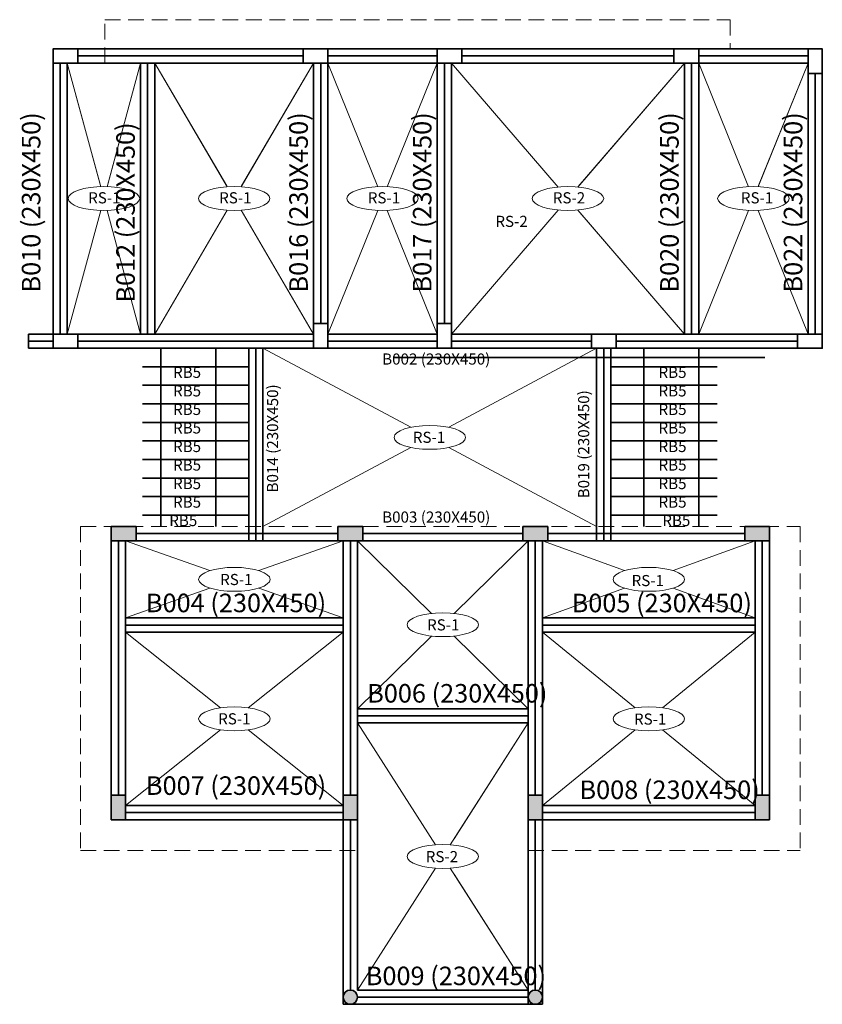
# Model space of a CAD drawing. Units: millimetres. Extents: x 15 to 330868, y -4710 to 1734924.
# Tile 1 of 3: x 280070 to 293056, y 850107 to 866041. Entities that reach past the tile are written whole.
import ezdxf

# ---------------------------------------------------------------- set-up
doc = ezdxf.new("R2010")
doc.units = ezdxf.units.MM
doc.header["$MEASUREMENT"] = 0
doc.linetypes.add('DASHED', pattern=[19.05, 12.7, -6.35])
for name, color, linetype, lineweight in [('S-ANNO-SYMB', 2, 'Continuous', 18), ('S-ANNO-TEXT', 7, 'Continuous', 18), ('S-BEAM', 7, 'Continuous', 35), ('S-COLS', 8, 'Continuous', 35), ('S-SLAB', 8, 'Continuous', 13), ('S-SLAB-OVHD', 6, 'DASHED', 18)]:
    doc.layers.add(name, color=color, linetype=linetype, lineweight=lineweight)
doc.styles.get("Standard").update_dxf_attribs({"font": 'arial.ttf'})

msp = doc.modelspace()

# ---------------------------------------------------------------- hatches: boundary and pattern name
at = {"layer": 'S-COLS'}
h = msp.add_hatch(color=256, dxfattribs=at)
h.dxf.hatch_style = 1
h.paths.add_polyline_path([(288527.5, 853493.6), (288297.5, 853493.6), (288297.5, 853093.6), (288527.5, 853093.6)])
h.paths.add_polyline_path([(285535, 853493.6), (285305, 853493.6), (285305, 853093.6), (285535, 853093.6)])
h.paths.add_polyline_path([(292200.2, 853493.6), (291970.2, 853493.6), (291970.2, 853093.6), (292200.2, 853093.6)])
h.paths.add_polyline_path([(288612.5, 857838.6), (288212.5, 857838.6), (288212.5, 857608.6), (288612.5, 857608.6)])
h.paths.add_polyline_path([(285620, 857838.6), (285220, 857838.6), (285220, 857608.6), (285620, 857608.6)])
h.paths.add_polyline_path([(281952, 857838.6), (281552, 857838.6), (281552, 857608.6), (281952, 857608.6)])
h.paths.add_polyline_path([(281782, 853493.6), (281552, 853493.6), (281552, 853093.6), (281782, 853093.6)])
h = msp.add_hatch(color=256, dxfattribs=at)
h.dxf.hatch_style = 1
h.paths.add_polyline_path([(292200.2, 857838.6), (291800.2, 857838.6), (291800.2, 857608.6), (292200.2, 857608.6)])
h = msp.add_hatch(color=256, dxfattribs=at)
h.dxf.hatch_style = 1
h.paths.add_polyline_path([(288527.5, 850221.5, 1), (288297.5, 850221.5, 1)])
h.paths.add_polyline_path([(285305, 850221.5, 1), (285535, 850221.5, 1)])

# ---------------------------------------------------------------- linework, layer by layer
at = {"layer": 'S-ANNO-SYMB'}
for centre in [(281433.2, 863146.1), (283540.7, 863146.1), (285940.7, 863146.1), (288940.7, 863146.1), (291940.7, 863146.1), (286705.4, 859281.1), (283543.5, 856983.7), (290248.8, 856983.7), (286916.3, 856249.6), (283543.5, 854726.2), (290248.8, 854726.2), (286916.3, 852498.6)]:
    msp.add_ellipse(centre, major_axis=(578.3, 0), ratio=0.3340635, dxfattribs=at)
at = {"layer": 'S-BEAM'}
for p, q in [((280610.7, 865568.6), (280610.7, 860723.6)), ((280610.7, 865568.6), (293055.7, 865568.6)), ((285055.7, 865568.6), (285055.7, 860723.6)), ((286825.7, 865568.6), (286825.7, 860723.6)), ((291055.7, 865568.6), (291055.7, 860953.6)), ((292825.7, 865568.6), (292825.7, 860953.6)), ((293055.7, 865568.6), (293055.7, 860723.6)), ((281010.7, 865453.6), (284655.7, 865453.6)), ((285055.7, 865453.6), (286825.7, 865453.6)), ((287225.7, 865453.6), (290655.7, 865453.6)), ((291055.7, 865453.6), (292825.7, 865453.6)), ((280610.7, 865338.6), (292825.7, 865338.6)), ((280725.7, 860953.6), (280725.7, 865338.6)), ((280840.7, 865338.6), (280840.7, 860953.6)), ((282025.7, 865338.6), (282025.7, 860953.6)), ((282140.7, 865338.6), (282140.7, 860953.6)), ((282255.7, 865338.6), (282255.7, 860953.6)), ((284825.7, 865338.6), (284825.7, 860723.6)), ((284940.7, 865338.6), (284940.7, 861123.6)), ((286940.7, 865338.6), (286940.7, 861123.6)), ((287055.7, 865338.6), (287055.7, 860723.6)), ((290825.7, 865338.6), (290825.7, 860953.6)), ((290940.7, 865338.6), (290940.7, 860953.6)), ((292940.7, 865168.6), (292940.7, 860953.6)), ((280210.7, 860953.6), (284825.7, 860953.6)), ((280210.7, 860953.6), (280210.7, 860723.6)), ((285055.7, 860953.6), (286825.7, 860953.6)), ((287055.7, 860953.6), (293055.7, 860953.6)), ((280610.7, 860838.6), (280210.7, 860838.6)), ((281010.7, 860838.6), (284825.7, 860838.6)), ((285055.7, 860838.6), (286825.7, 860838.6)), ((287055.7, 860838.6), (289319.1, 860838.6)), ((289719.1, 860838.6), (292655.7, 860838.6)), ((280210.7, 860723.6), (293055.7, 860723.6)), ((282354.7, 860723.6), (282354.7, 857838.6)), ((283241.3, 860723.6), (283241.3, 857838.6)), ((283776.6, 860723.6), (283776.6, 857608.6)), ((283891.6, 860723.6), (283891.6, 857608.6)), ((284006.6, 860723.6), (284006.6, 857608.6)), ((289404.1, 860723.6), (289404.1, 857608.6)), ((289519.1, 860723.6), (289519.1, 857608.6)), ((289634.1, 860723.6), (289634.1, 857608.6)), ((290169.2, 860723.6), (290169.2, 857838.6)), ((291055.7, 860723.6), (291055.7, 857838.6)), ((286126.6, 860572.5), (292126.6, 860572.5)), ((283776.4, 860423.6), (282054.7, 860423.6)), ((289634.1, 860423.6), (291355.7, 860423.6)), ((283776.4, 860123.6), (282054.7, 860123.6)), ((289634.1, 860123.6), (291355.7, 860123.6)), ((283776.4, 859823.6), (282054.7, 859823.6)), ((289634.1, 859823.6), (291355.7, 859823.6)), ((283776.4, 859523.6), (282054.7, 859523.6)), ((289634.1, 859523.6), (291355.7, 859523.6)), ((283776.4, 859223.6), (282054.7, 859223.6)), ((289634.1, 859223.6), (291355.7, 859223.6)), ((283776.4, 858923.6), (282054.7, 858923.6)), ((289634.1, 858923.6), (291355.7, 858923.6)), ((283776.4, 858623.6), (282054.7, 858623.6)), ((289634.1, 858623.6), (291355.7, 858623.6)), ((283776.4, 858323.6), (282054.7, 858323.6)), ((289634.1, 858323.6), (291355.7, 858323.6)), ((283776.4, 858023.6), (282054.7, 858023.6)), ((289634.1, 858023.6), (291355.7, 858023.6)), ((281552, 857838.6), (281552, 853093.6)), ((292200.2, 857838.6), (292200.2, 853093.6)), ((281552, 857608.6), (292200.2, 857608.6)), ((281667, 857608.6), (281667, 853493.6)), ((281782, 857608.6), (281782, 853093.6)), ((281952, 857723.6), (285220, 857723.6)), ((285305, 857608.6), (285305, 850106.5)), ((285420, 857608.6), (285420, 853493.6)), ((285535, 857608.6), (285535, 850336.5)), ((285620, 857723.6), (288212.5, 857723.6)), ((288297.5, 857608.6), (288297.5, 850106.5)), ((288412.5, 857608.6), (288412.5, 853493.6)), ((288527.5, 857608.6), (288527.5, 850106.5)), ((288612.5, 857723.6), (291800.2, 857723.6)), ((291970.2, 857608.6), (291970.2, 853093.6)), ((292085.2, 857608.6), (292085.2, 853493.6)), ((281782, 856358.9), (285305, 856358.9)), ((288527.5, 856358.9), (291970.2, 856358.9)), ((281782, 856243.9), (285305, 856243.9)), ((288527.5, 856243.9), (291970.2, 856243.9)), ((281782, 856128.9), (285305, 856128.9)), ((288527.5, 856128.9), (291970.2, 856128.9)), ((285535, 854890.7), (288297.5, 854890.7)), ((285535, 854775.7), (288297.5, 854775.7)), ((285535, 854660.7), (288297.5, 854660.7)), ((281782, 853323.6), (285305, 853323.6)), ((288527.5, 853323.6), (291970.2, 853323.6)), ((281782, 853208.6), (285305, 853208.6)), ((288527.5, 853208.6), (291970.2, 853208.6)), ((281552, 853093.6), (285535, 853093.6)), ((285420, 853093.6), (285420, 850336.5)), ((288297.5, 853093.6), (292200.2, 853093.6)), ((288412.5, 853093.6), (288412.5, 850336.5)), ((285535, 850336.5), (288297.5, 850336.5)), ((285305, 850106.5), (288527.5, 850106.5)), ((285535, 850221.5), (288297.5, 850221.5))]:
    msp.add_line(p, q, dxfattribs=at)
for points in [[(281010.7, 865568.6), (281010.7, 865338.6), (280610.7, 865338.6), (280610.7, 865568.6)], [(285055.7, 865568.6), (285055.7, 865338.6), (284655.7, 865338.6), (284655.7, 865568.6)], [(287225.7, 865568.6), (287225.7, 865338.6), (286825.7, 865338.6), (286825.7, 865568.6)], [(291055.7, 865568.6), (291055.7, 865338.6), (290655.7, 865338.6), (290655.7, 865568.6)], [(292825.7, 865568.6), (293055.7, 865568.6), (293055.7, 865168.6), (292825.7, 865168.6)], [(284825.7, 861123.6), (285055.7, 861123.6), (285055.7, 860723.6), (284825.7, 860723.6)], [(286825.7, 861123.6), (287055.7, 861123.6), (287055.7, 860723.6), (286825.7, 860723.6)], [(281010.7, 860953.6), (281010.7, 860723.6), (280610.7, 860723.6), (280610.7, 860953.6)], [(289719.1, 860953.6), (289719.1, 860723.6), (289319.1, 860723.6), (289319.1, 860953.6)], [(293055.7, 860953.6), (293055.7, 860723.6), (292655.7, 860723.6), (292655.7, 860953.6)], [(281952, 857838.6), (281952, 857608.6), (281552, 857608.6), (281552, 857838.6)], [(285620, 857838.6), (285620, 857608.6), (285220, 857608.6), (285220, 857838.6)], [(288612.5, 857838.6), (288612.5, 857608.6), (288212.5, 857608.6), (288212.5, 857838.6)], [(292200.2, 857838.6), (292200.2, 857608.6), (291800.2, 857608.6), (291800.2, 857838.6)], [(281552, 853493.6), (281782, 853493.6), (281782, 853093.6), (281552, 853093.6)], [(285305, 853493.6), (285535, 853493.6), (285535, 853093.6), (285305, 853093.6)], [(288297.5, 853493.6), (288527.5, 853493.6), (288527.5, 853093.6), (288297.5, 853093.6)], [(291970.2, 853493.6), (292200.2, 853493.6), (292200.2, 853093.6), (291970.2, 853093.6)]]:
    msp.add_lwpolyline(points, close=True, dxfattribs=at)
at = {"layer": 'S-COLS'}
for centre in [(285420, 850221.5), (288412.5, 850221.5)]:
    msp.add_circle(centre, 115, dxfattribs=at)
at = {"layer": 'S-SLAB'}
for p, q in [((281375.7, 863358.9), (280840.7, 865338.6)), ((281381.2, 863338.5), (280840.7, 865338.6)), ((282025.7, 865338.6), (281485.2, 863338.5)), ((282025.7, 865338.6), (281490.8, 863358.9)), ((282255.7, 865338.6), (283421.2, 863350.1)), ((282255.7, 865338.6), (283429.6, 863335.7)), ((283651.9, 863335.7), (284825.7, 865338.6)), ((283660.3, 863350.1), (284825.7, 865338.6)), ((285055.7, 865338.6), (285864.4, 863335.1)), ((286016.3, 863333.3), (286825.7, 865338.6)), ((287055.7, 865338.6), (288781.1, 863331.8)), ((289100.4, 863331.8), (290825.7, 865338.6)), ((289106.4, 863338.8), (290825.7, 865338.6)), ((291055.7, 865338.6), (291863.5, 863337.6)), ((292018, 863337.6), (292825.7, 865338.6)), ((292025.4, 863355.9), (292825.7, 865338.6)), ((281381.2, 862953.7), (280840.7, 860953.6)), ((282025.7, 860953.6), (281485.2, 862953.7)), ((282255.7, 860953.6), (283429.6, 862956.5)), ((283651.9, 862956.5), (284825.7, 860953.6)), ((285055.7, 860953.6), (285863.5, 862954.7)), ((286018, 862954.7), (286825.7, 860953.6)), ((287055.7, 860953.6), (288781.1, 862960.4)), ((289100.4, 862960.4), (290825.7, 860953.6)), ((289106.4, 862953.4), (290825.7, 860953.6)), ((291055.7, 860953.6), (291863.5, 862954.7)), ((292018, 862954.7), (292825.7, 860953.6)), ((284006.6, 860723.6), (286398.9, 859444.9)), ((289404.1, 860723.6), (287011.9, 859444.9)), ((286398.9, 859117.3), (284006.6, 857838.6)), ((287011.9, 859117.3), (289404.1, 857838.6)), ((281782, 857608.6), (283147, 857124.4)), ((283940, 857124.4), (285305, 857608.6)), ((285535, 857608.6), (286730.3, 856432.6)), ((287102.2, 856432.6), (288297.5, 857608.6)), ((289857.3, 857125.9), (288527.5, 857608.6)), ((290640.4, 857125.9), (291970.2, 857608.6)), ((281782, 856358.9), (283147, 856843.1)), ((283940, 856843.1), (285305, 856358.9)), ((288527.5, 856358.9), (289857.3, 856841.6)), ((291970.2, 856358.9), (290640.4, 856841.6)), ((283319.8, 854904.4), (281782, 856128.9)), ((283767.2, 854904.4), (285305, 856128.9)), ((285535, 854890.7), (286730.3, 856066.7)), ((287102.2, 856066.7), (288297.5, 854890.7)), ((288527.5, 856128.9), (290029.5, 854905)), ((291970.2, 856128.9), (290468.2, 854905)), ((285535, 854660.7), (286795.5, 852687.5)), ((287037, 852687.5), (288297.5, 854660.7)), ((287097.5, 852782.4), (288297.5, 854660.7)), ((281782, 853323.6), (283319.8, 854548.1)), ((285305, 853323.6), (283767.2, 854548.1)), ((290029.5, 854547.5), (288527.5, 853323.6)), ((290468.2, 854547.5), (291970.2, 853323.6)), ((285535, 850336.5), (286795.5, 852309.7)), ((287037, 852309.7), (288297.5, 850336.5)), ((287099.9, 852211.2), (288297.5, 850336.5))]:
    msp.add_line(p, q, dxfattribs=at)
at = {"layer": 'S-SLAB-OVHD', "ltscale": 20}
for p, q in [((281445.5, 865338.6), (281445.5, 866040.7)), ((281445.5, 866040.7), (291564.7, 866040.7)), ((291564.7, 866040.7), (291564.7, 865568.6)), ((281052, 857838.6), (292700.2, 857838.6)), ((281052, 857838.6), (281052, 852593.6)), ((292700.2, 857838.6), (292700.2, 852593.6)), ((281052, 852593.6), (285535, 852593.6)), ((288297.5, 852593.6), (292700.2, 852593.6))]:
    msp.add_line(p, q, dxfattribs=at)

# ---------------------------------------------------------------- texts
at = {"layer": 'S-ANNO-TEXT', "attachment_point": 1, "rotation": 90}
for s, width, insert, char_height in [('\\pxt0,1;B010 (230X450)', 4992.481, (280105.1, 861625.9), 300), ('\\pxt0,1;B016 (230X450)', 4992.481, (284432.4, 861625.9), 300), ('\\pxt0,1;B017 (230X450)', 4992.481, (286432.4, 861625.9), 300), ('\\pxt0,1;B020 (230X450)', 4992.481, (290432.4, 861625.9), 300), ('\\pxt0,1;B022 (230X450)', 4992.481, (292432.4, 861625.9), 300), ('\\pxt0,1;B012 (230X450)', 4992.481, (281632.4, 861462.5), 300), ('\\pxt0;B014 (230X450)', 2161.345, (284071.4, 858390.2), 180), ('B019 (230X450)', 2161.345, (289104.9, 858294.7), 180)]:
    msp.add_mtext_dynamic_manual_height_columns(s, width=width, gutter_width=1, heights=[0], dxfattribs=dict(at, insert=insert, char_height=char_height))
at = {"layer": 'S-ANNO-TEXT'}
for s, width, insert, char_height, attachment_point in [('RS-1', 774.454, (281178.2, 863248.3), 180, 1), ('RS-1', 774.454, (283297.3, 863248.3), 180, 1), ('RS-1', 774.454, (285702, 863248.3), 180, 1), ('RS-2', 774.454, (288695.6, 863248.3), 180, 1), ('RS-1', 774.454, (291738, 863248.3), 180, 1), ('RS-2', 774.454, (287766.4, 862867.2), 180, 1), ('B002 (230X450)', 2161.345, (285934.7, 860639.2), 180, 1), ('RB5 ', 774.454, (283005, 860423.6), 180, 3), ('RB5 ', 774.454, (290405.5, 860423.6), 180, 1), ('RB5 ', 774.454, (283005, 860123.6), 180, 3), ('RB5 ', 774.454, (290405.5, 860123.6), 180, 1), ('RB5 ', 774.454, (283005, 859823.6), 180, 3), ('RB5 ', 774.454, (290405.5, 859823.6), 180, 1), ('RB5 ', 774.454, (283005, 859523.6), 180, 3), ('RB5 ', 774.454, (290405.5, 859523.6), 180, 1), ('RS-1', 774.454, (286430.7, 859372.5), 180, 1), ('RB5 ', 774.454, (283005, 859223.6), 180, 3), ('RB5 ', 774.454, (290405.5, 859223.6), 180, 1), ('RB5 ', 774.454, (283005, 858923.6), 180, 3), ('RB5 ', 774.454, (290405.5, 858923.6), 180, 1), ('RB5 ', 774.454, (283005, 858623.6), 180, 3), ('RB5 ', 774.454, (290405.5, 858623.6), 180, 1), ('RB5 ', 774.454, (283005, 858323.6), 180, 3), ('RB5 ', 774.454, (290405.5, 858323.6), 180, 1), ('B003 (230X450)', 2161.345, (285934.7, 858081.8), 180, 1), ('RB5 ', 774.454, (282943.4, 858025.1), 180, 3), ('RB5 ', 774.454, (290467.1, 858025.1), 180, 1), ('RS-1', 774.454, (283313.4, 857071), 180, 1), ('RS-1', 774.454, (289970.6, 857054), 180, 1), ('\\pxt0,1;B004 (230X450)', 4992.481, (282112.8, 856752), 300, 1), ('\\pxt0,1;B005 (230X450)', 4992.481, (289000.8, 856751), 300, 1), ('RS-1', 774.454, (286661.3, 856337.2), 180, 1), ('\\pxt0,1;B006 (230X450)', 4992.481, (285692.5, 855289.5), 300, 1), ('RS-1', 774.454, (283281.3, 854816.7), 180, 1), ('RS-1', 774.454, (290008.7, 854812.7), 180, 1), ('\\pxt0,1;B007 (230X450)', 4992.481, (282112.8, 853795.7), 300, 1), ('\\pxt0,1;B008 (230X450)', 4992.481, (289127.2, 853728.2), 300, 1), ('RS-2', 774.454, (286639.3, 852586.2), 180, 1), ('\\pxt0,1;B009 (230X450)', 4992.481, (285670.4, 850716.3), 300, 1)]:
    msp.add_mtext_dynamic_manual_height_columns(s, width=width, gutter_width=1, heights=[0], dxfattribs=dict(at, insert=insert, char_height=char_height, attachment_point=attachment_point))

doc.saveas('drawing.dxf')
